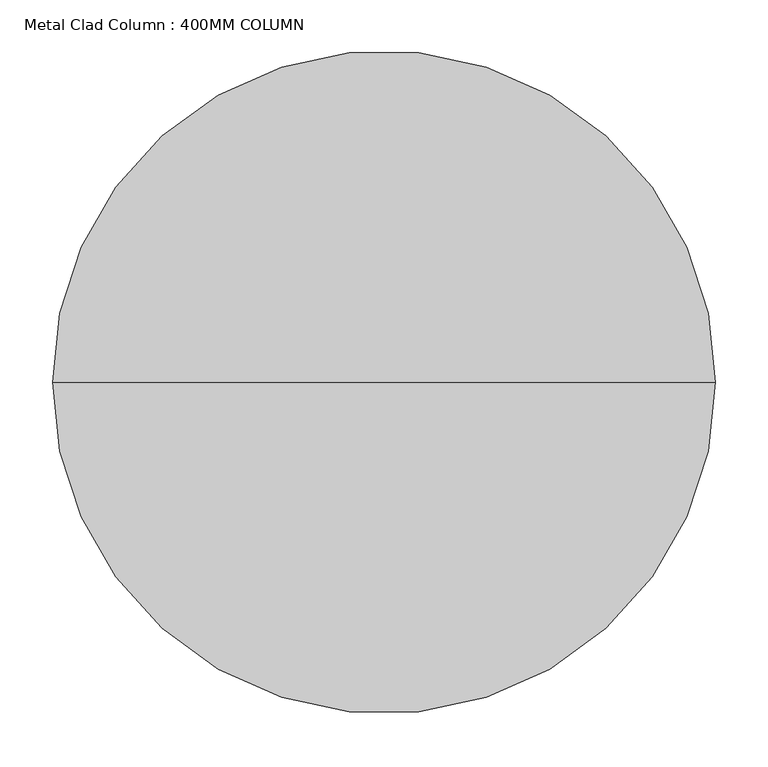
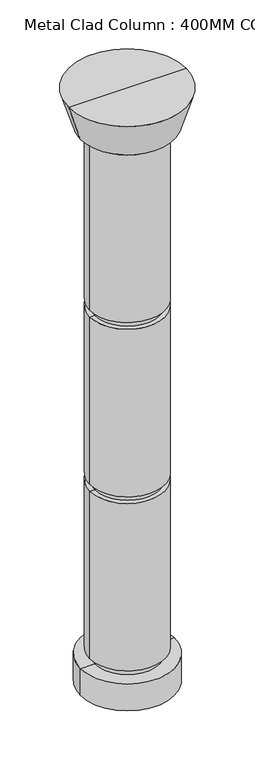
"""IFC4 building model written with IfcOpenShell, lengths in millimetres: column geometry, Metal Clad Column : 400MM COLUMN."""

from ifc_helpers import new_model, si_unit, frame, origin, place, context, project, spatial, polyline, circle_curve, source, transform, mapped, element, save
from ifc_brep_helpers import plane_surface, cylinder_surface, revolved_surface, advanced_brep


def metal_clad_column_400mm_column_f648cdbd(model_context):
    return source(origin(), model_context, "Body", "AdvancedBrep", [
        advanced_brep(
        [(0.0, 0.0, -100.0), (-250.8, 0.0, -100.0), (250.8, 0.0, -100.0), (-250.8, 0.0, 52.4), (250.8, 0.0, 52.4), (174.6, 0.0, 1075.9333333), (-174.6, 0.0, 1075.9333333), (-200.0, 0.0, 1075.9333333), (200.0, 0.0, 1075.9333333), (-200.0, 0.0, 2023.2666667), (200.0, 0.0, 2023.2666667), (174.6, 0.0, 1037.8333333), (-174.6, 0.0, 1037.8333333), (200.0, 0.0, 1037.8333333), (-200.0, 0.0, 1037.8333333), (200.0, 0.0, 90.5), (-200.0, 0.0, 90.5), (174.6, 0.0, 90.5), (-174.6, 0.0, 90.5), (174.6, 0.0, 52.4), (-174.6, 0.0, 52.4), (250.8, 0.0, 3046.8), (-250.8, 0.0, 3046.8), (-314.3, 0.0, 3250.0), (314.3, 0.0, 3250.0), (0.0, 0.0, 3250.0), (174.6, 0.0, 3046.8), (-174.6, 0.0, 3046.8), (174.6, 0.0, 3008.7), (-174.6, 0.0, 3008.7), (200.0, 0.0, 3008.7), (-200.0, 0.0, 3008.7), (200.0, 0.0, 2061.3666667), (-200.0, 0.0, 2061.3666667), (174.6, 0.0, 2061.3666667), (-174.6, 0.0, 2061.3666667), (174.6, 0.0, 2023.2666667), (-174.6, 0.0, 2023.2666667)],
        [
            (0, 1),
            (1, 2, circle_curve(frame((0.0, 0.0, -100.0), z_axis=(0.0, 0.0, -1.0), x_axis=(-1.0, 0.0, 0.0)), 250.8)),
            (2, 0),
            (2, 1, circle_curve(frame((0.0, 0.0, -100.0), z_axis=(0.0, 0.0, -1.0), x_axis=(-1.0, 0.0, 0.0)), 250.8)),
            (1, 3),
            (3, 4, circle_curve(frame((0.0, 0.0, 52.4), z_axis=(0.0, 0.0, -1.0), x_axis=(-1.0, 0.0, 0.0)), 250.8)),
            (4, 2),
            (4, 3, circle_curve(frame((0.0, 0.0, 52.4), z_axis=(0.0, 0.0, -1.0), x_axis=(-1.0, 0.0, 0.0)), 250.8)),
            (5, 6, circle_curve(frame((0.0, 0.0, 1075.9333333), z_axis=(0.0, 0.0, 1.0), x_axis=(-1.0, 0.0, 0.0)), 174.6)),
            (6, 7),
            (7, 8, circle_curve(frame((0.0, 0.0, 1075.9333333), z_axis=(0.0, 0.0, -1.0), x_axis=(-1.0, 0.0, 0.0)), 200.0)),
            (8, 5),
            (7, 9),
            (9, 10, circle_curve(frame((0.0, 0.0, 2023.2666667), z_axis=(0.0, 0.0, -1.0), x_axis=(-1.0, 0.0, 0.0)), 200.0)),
            (10, 8),
            (7, 8, circle_curve(frame((0.0, 0.0, 1075.9333333), z_axis=(0.0, 0.0, 1.0), x_axis=(-1.0, 0.0, 0.0)), 200.0)),
            (10, 9, circle_curve(frame((0.0, 0.0, 2023.2666667), z_axis=(0.0, 0.0, -1.0), x_axis=(-1.0, 0.0, 0.0)), 200.0)),
            (6, 5, circle_curve(frame((0.0, 0.0, 1075.9333333), z_axis=(0.0, 0.0, 1.0), x_axis=(-1.0, 0.0, 0.0)), 174.6)),
            (11, 12, circle_curve(frame((0.0, 0.0, 1037.8333333), z_axis=(0.0, 0.0, 1.0), x_axis=(-1.0, 0.0, 0.0)), 174.6)),
            (12, 6),
            (5, 11),
            (12, 11, circle_curve(frame((0.0, 0.0, 1037.8333333), z_axis=(0.0, 0.0, 1.0), x_axis=(-1.0, 0.0, 0.0)), 174.6)),
            (13, 14, circle_curve(frame((0.0, 0.0, 1037.8333333), z_axis=(0.0, 0.0, 1.0), x_axis=(-1.0, 0.0, 0.0)), 200.0)),
            (14, 12),
            (11, 13),
            (14, 13, circle_curve(frame((0.0, 0.0, 1037.8333333), z_axis=(0.0, 0.0, 1.0), x_axis=(-1.0, 0.0, 0.0)), 200.0)),
            (15, 16, circle_curve(frame((0.0, 0.0, 90.5), z_axis=(0.0, 0.0, 1.0), x_axis=(-1.0, 0.0, 0.0)), 200.0)),
            (16, 14),
            (13, 15),
            (16, 15, circle_curve(frame((0.0, 0.0, 90.5), z_axis=(0.0, 0.0, 1.0), x_axis=(-1.0, 0.0, 0.0)), 200.0)),
            (17, 18, circle_curve(frame((0.0, 0.0, 90.5), z_axis=(0.0, 0.0, 1.0), x_axis=(-1.0, 0.0, 0.0)), 174.6)),
            (18, 16),
            (15, 17),
            (18, 17, circle_curve(frame((0.0, 0.0, 90.5), z_axis=(0.0, 0.0, 1.0), x_axis=(-1.0, 0.0, 0.0)), 174.6)),
            (19, 20, circle_curve(frame((0.0, 0.0, 52.4), z_axis=(0.0, 0.0, 1.0), x_axis=(-1.0, 0.0, 0.0)), 174.6)),
            (20, 18),
            (17, 19),
            (20, 19, circle_curve(frame((0.0, 0.0, 52.4), z_axis=(0.0, 0.0, 1.0), x_axis=(-1.0, 0.0, 0.0)), 174.6)),
            (3, 20),
            (19, 4),
            (21, 22, circle_curve(frame((0.0, 0.0, 3046.8), z_axis=(0.0, 0.0, 1.0), x_axis=(-1.0, 0.0, 0.0)), 250.8)),
            (22, 23),
            (23, 24, circle_curve(frame((0.0, 0.0, 3250.0), z_axis=(0.0, 0.0, -1.0), x_axis=(-1.0, 0.0, 0.0)), 314.3)),
            (24, 21),
            (23, 25),
            (25, 24),
            (23, 24, circle_curve(frame((0.0, 0.0, 3250.0), z_axis=(0.0, 0.0, 1.0), x_axis=(-1.0, 0.0, 0.0)), 314.3)),
            (22, 21, circle_curve(frame((0.0, 0.0, 3046.8), z_axis=(0.0, 0.0, 1.0), x_axis=(-1.0, 0.0, 0.0)), 250.8)),
            (26, 27, circle_curve(frame((0.0, 0.0, 3046.8), z_axis=(0.0, 0.0, 1.0), x_axis=(-1.0, 0.0, 0.0)), 174.6)),
            (27, 22),
            (21, 26),
            (27, 26, circle_curve(frame((0.0, 0.0, 3046.8), z_axis=(0.0, 0.0, 1.0), x_axis=(-1.0, 0.0, 0.0)), 174.6)),
            (28, 29, circle_curve(frame((0.0, 0.0, 3008.7), z_axis=(0.0, 0.0, 1.0), x_axis=(-1.0, 0.0, 0.0)), 174.6)),
            (29, 27),
            (26, 28),
            (29, 28, circle_curve(frame((0.0, 0.0, 3008.7), z_axis=(0.0, 0.0, 1.0), x_axis=(-1.0, 0.0, 0.0)), 174.6)),
            (30, 31, circle_curve(frame((0.0, 0.0, 3008.7), z_axis=(0.0, 0.0, 1.0), x_axis=(-1.0, 0.0, 0.0)), 200.0)),
            (31, 29),
            (28, 30),
            (31, 30, circle_curve(frame((0.0, 0.0, 3008.7), z_axis=(0.0, 0.0, 1.0), x_axis=(-1.0, 0.0, 0.0)), 200.0)),
            (32, 33, circle_curve(frame((0.0, 0.0, 2061.3666667), z_axis=(0.0, 0.0, 1.0), x_axis=(-1.0, 0.0, 0.0)), 200.0)),
            (33, 31),
            (30, 32),
            (33, 32, circle_curve(frame((0.0, 0.0, 2061.3666667), z_axis=(0.0, 0.0, 1.0), x_axis=(-1.0, 0.0, 0.0)), 200.0)),
            (34, 35, circle_curve(frame((0.0, 0.0, 2061.3666667), z_axis=(0.0, 0.0, 1.0), x_axis=(-1.0, 0.0, 0.0)), 174.6)),
            (35, 33),
            (32, 34),
            (35, 34, circle_curve(frame((0.0, 0.0, 2061.3666667), z_axis=(0.0, 0.0, 1.0), x_axis=(-1.0, 0.0, 0.0)), 174.6)),
            (36, 37, circle_curve(frame((0.0, 0.0, 2023.2666667), z_axis=(0.0, 0.0, 1.0), x_axis=(-1.0, 0.0, 0.0)), 174.6)),
            (37, 35),
            (34, 36),
            (37, 36, circle_curve(frame((0.0, 0.0, 2023.2666667), z_axis=(0.0, 0.0, 1.0), x_axis=(-1.0, 0.0, 0.0)), 174.6)),
            (9, 37),
            (36, 10),
        ],
        [
            plane_surface(frame((0.0, 0.0, -100.0), z_axis=(0.0, 0.0, -1.0), x_axis=(-1.0, 0.0, 0.0))),
            cylinder_surface(frame((0.0, 0.0, 3250.0), z_axis=(0.0, 0.0, -1.0), x_axis=(-1.0, 0.0, 0.0)), 250.8),
            plane_surface(frame((0.0, 0.0, 1075.9333333), z_axis=(0.0, 0.0, -1.0), x_axis=(-1.0, 0.0, 0.0))),
            cylinder_surface(frame((0.0, 0.0, 3250.0), z_axis=(0.0, 0.0, -1.0), x_axis=(-1.0, 0.0, 0.0)), 200.0),
            cylinder_surface(frame((0.0, 0.0, 3250.0), z_axis=(0.0, 0.0, -1.0), x_axis=(-1.0, 0.0, 0.0)), 174.6),
            plane_surface(frame((0.0, 0.0, 1037.8333333), z_axis=(0.0, 0.0, 1.0), x_axis=(-1.0, 0.0, 0.0))),
            plane_surface(frame((0.0, 0.0, 90.5), z_axis=(0.0, 0.0, -1.0), x_axis=(-1.0, 0.0, 0.0))),
            plane_surface(frame((0.0, 0.0, 52.4), z_axis=(0.0, 0.0, 1.0), x_axis=(-1.0, 0.0, 0.0))),
            revolved_surface(polyline([(-314.3, 0.0, 3250.0), (-250.8, 0.0, 3046.8)]), (0.0, 0.0, 3250.0), (0.0, 0.0, -1.0)),
            plane_surface(frame((0.0, 0.0, 3250.0), z_axis=(0.0, 0.0, 1.0), x_axis=(-1.0, 0.0, 0.0))),
            plane_surface(frame((0.0, 0.0, 3046.8), z_axis=(0.0, 0.0, -1.0), x_axis=(-1.0, 0.0, 0.0))),
            plane_surface(frame((0.0, 0.0, 3008.7), z_axis=(0.0, 0.0, 1.0), x_axis=(-1.0, 0.0, 0.0))),
            plane_surface(frame((0.0, 0.0, 2061.3666667), z_axis=(0.0, 0.0, -1.0), x_axis=(-1.0, 0.0, 0.0))),
            plane_surface(frame((0.0, 0.0, 2023.2666667), z_axis=(0.0, 0.0, 1.0), x_axis=(-1.0, 0.0, 0.0))),
        ],
        [
            (0, [[1, 2, 3]]),
            (0, [[-3, 4, -1]]),
            (1, [[-2, 5, 6, 7]]),
            (1, [[-4, -7, 8, -5]]),
            (2, [[9, 10, 11, 12]]),
            (3, [[-11, 13, 14, 15]]),
            (3, [[16, -15, 17, -13]]),
            (2, [[18, -12, -16, -10]]),
            (4, [[19, 20, -9, 21]]),
            (4, [[22, -21, -18, -20]]),
            (5, [[23, 24, -19, 25]]),
            (5, [[26, -25, -22, -24]]),
            (3, [[27, 28, -23, 29]]),
            (3, [[30, -29, -26, -28]]),
            (6, [[31, 32, -27, 33]]),
            (6, [[34, -33, -30, -32]]),
            (4, [[35, 36, -31, 37]]),
            (4, [[38, -37, -34, -36]]),
            (7, [[-6, 39, -35, 40]]),
            (7, [[-8, -40, -38, -39]]),
            (8, [[41, 42, 43, 44]]),
            (9, [[-43, 45, 46]]),
            (9, [[47, -46, -45]]),
            (8, [[48, -44, -47, -42]]),
            (10, [[49, 50, -41, 51]]),
            (10, [[52, -51, -48, -50]]),
            (4, [[53, 54, -49, 55]]),
            (4, [[56, -55, -52, -54]]),
            (11, [[57, 58, -53, 59]]),
            (11, [[60, -59, -56, -58]]),
            (3, [[61, 62, -57, 63]]),
            (3, [[64, -63, -60, -62]]),
            (12, [[65, 66, -61, 67]]),
            (12, [[68, -67, -64, -66]]),
            (4, [[69, 70, -65, 71]]),
            (4, [[72, -71, -68, -70]]),
            (13, [[-14, 73, -69, 74]]),
            (13, [[-17, -74, -72, -73]]),
        ],
    ),
    ])


if __name__ == "__main__":
    model = new_model("IFC4")
    model_context = context("Model", 3, world=origin())
    ifc_project = project(units=[si_unit("LENGTHUNIT", "METRE", prefix="MILLI")], contexts=[model_context])
    site = spatial("IfcSite", under=ifc_project)
    building = spatial("IfcBuilding", under=site)
    placement = place(None, origin())
    metal_clad_column_400mm_column_shape = metal_clad_column_400mm_column_f648cdbd(model_context)
    element("IfcColumn", 1, ObjectType="Metal Clad Column : 400MM COLUMN", at=placement, inside=building, context=model_context, shape_type="MappedRepresentation", body=[
        mapped(metal_clad_column_400mm_column_shape, transform((0.0, 0.0, 0.0), x_axis=(1.0, 0.0, 0.0), y_axis=(0.0, 1.0, 0.0), z_axis=(0.0, 0.0, 1.0))),
    ])
    save(model, "model.ifc")

# Revit data of these elements
# Type "Metal Clad Column : 400MM COLUMN"
#   Assembly Code = "B1010200"
#   Base = 0' - 6"
#   Capital = 0' - 8"
#   Diameter = 1' - 3.74803"
#   Joint Depth = 0' - 1"
#   Joint Width = 0' - 1 1/2"
#   Offset base level = 0' - 0"
#   Offset top level = 0' - 0"
#   Material = Aluminum
# Element 1 (IfcColumn, "Metal Clad Column : 400MM COLUMN")
#   Materials on its faces: "Aluminum"
# Materials
#   "Aluminum": class "Metal", colour RGB 247 247 247, transparency 0, Description = "Aluminum 6061", Cost = 0
